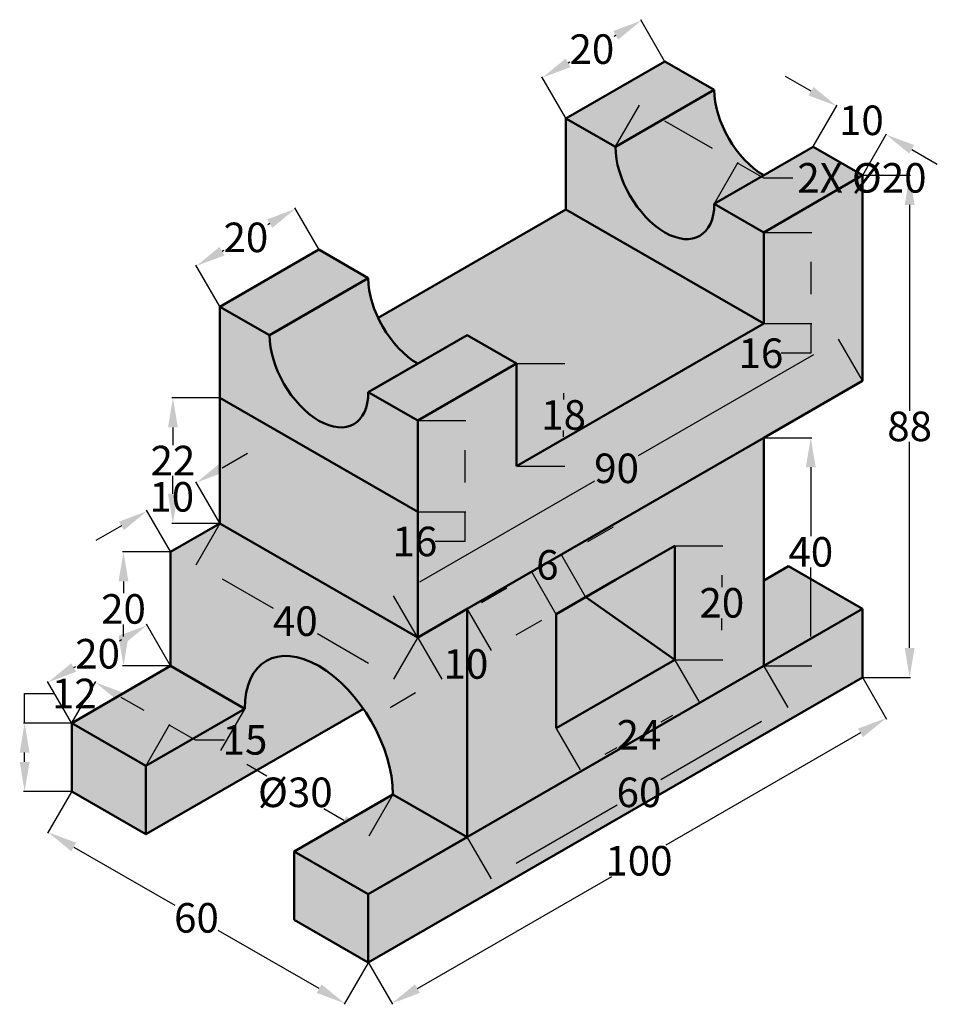
# Model space of a CAD drawing. Units: millimetres. Extents: x 125 to 286, y 8 to 181.
import ezdxf

# ---------------------------------------------------------------- set-up
doc = ezdxf.new("R2010")
doc.units = ezdxf.units.MM
doc.header["$MEASUREMENT"] = 0
for name, color, linetype, lineweight in [('M-DIMS', 2, 'Continuous', 18), ('M-HATC', 252, 'Continuous', 18), ('M-OUTL', 7, 'Continuous', 50)]:
    doc.layers.add(name, color=color, linetype=linetype, lineweight=lineweight)
doc.styles.get("Standard").update_dxf_attribs({"font": 'arial.ttf'})
doc.dimstyles.get("Standard").update_dxf_attribs({"dimtxt": 5.179999999999999, "dimasz": 5.179999999999999, "dimexe": 0.18, "dimexo": 0.0625, "dimgap": 0.09, "dimtad": 0, "dimtih": 1, "dimtoh": 1, "dimdec": 1, "dimzin": 0, "dimdsep": 46, "dimtxsty": 'Standard', "dimcen": 0.09, "dimadec": 0, "dimazin": 0, "dimtfac": 1, "dimtdec": 1, "dimtofl": 0, "dimtmove": 0, "dimatfit": 3, "dimfxl": 1, "dimtolj": 1, "dimtzin": 0, "dimarcsym": 0})

# ---------------------------------------------------------------- blocks, each defined once
blk = doc.blocks.new('*D1')
at = {"layer": 'Defpoints', "color": 0, "transparency": 16777216}
for p in [(272.9292849999999, 65.249038), (186.326745, 15.24903799999998), (190.4517447010181, 8.104328936630097)]:
    blk.add_point(p, dxfattribs=at)
at = {"layer": 'M-DIMS', "color": 0, "lineweight": -2, "transparency": 16777216}
for p, q in [((272.9605349999999, 65.19491141226347), (277.1442847956291, 57.94844420007783)), ((272.5682732040257, 55.51432877275904), (238.489772003563, 35.83909693109291)), ((194.9377562926215, 10.6943289366301), (229.0162574930842, 30.36956077829619)), ((186.3579949999999, 15.19491141226346), (190.5417447010181, 7.94844436394888))]:
    blk.add_line(p, q, dxfattribs=at)
at = {"layer": 'M-DIMS', "color": 0, "transparency": 16777216}
for points in [[(272.1366065373591, 56.26199737135959), (272.9999398706924, 54.76666017415848), (277.0542847956291, 58.10432877275904)], [(194.5060896259549, 11.44199753523065), (195.3694229592882, 9.946660338029531), (190.4517447010181, 8.104328936630097)]]:
    blk.add_solid(points, dxfattribs=at)
at = {"layer": 'M-DIMS', "color": 0, "transparency": 16777216, "insert": (233.7530147483236, 33.10432885469456), "char_height": 5.179999999999999, "attachment_point": 5}
blk.add_mtext('\\A1;100', dxfattribs=at)
blk = doc.blocks.new('*D2')
at = {"layer": 'Defpoints', "color": 0, "transparency": 16777216}
for p in [(134.3652209999999, 45.24903799999999), (130.240221223293, 38.10432880553328), (186.326745, 15.24903800000001)]:
    blk.add_point(p, dxfattribs=at)
at = {"layer": 'M-DIMS', "color": 0, "lineweight": -2, "transparency": 16777216}
for p, q in [((134.3339709999999, 45.19491141226347), (130.150221223293, 37.94844423285206)), ((134.7262328148964, 35.51432880553328), (152.415587617297, 25.30137504857649)), ((177.7157336884562, 10.69432890385592), (160.0263788860555, 20.90728266081271)), ((186.2954949999999, 15.19491141226348), (182.1117452800596, 7.948444331174698))]:
    blk.add_line(p, q, dxfattribs=at)
at = {"layer": 'M-DIMS', "color": 0, "transparency": 16777216}
for points in [[(135.157899481563, 36.26199740413384), (134.2945661482297, 34.76666020693271), (130.240221223293, 38.10432880553328)], [(178.1474003551229, 11.44199750245647), (177.2840670217895, 9.94666030525535), (182.2017452800596, 8.104328903855915)]]:
    blk.add_solid(points, dxfattribs=at)
at = {"layer": 'M-DIMS', "color": 0, "transparency": 16777216, "insert": (156.2209832516763, 23.1043288546946), "char_height": 5.179999999999999, "attachment_point": 5}
blk.add_mtext('\\A1;60', dxfattribs=at)
blk = doc.blocks.new('*D3')
at = {"layer": 'Defpoints', "color": 0, "transparency": 16777216}
for p in [(134.365221, 57.24903799999999), (151.4806020634321, 56.89374769108934), (147.355602, 49.74903799999999)]:
    blk.add_point(p, dxfattribs=at)
at = {"layer": 'M-DIMS', "color": 0, "lineweight": -2, "transparency": 16777216}
for p, q in [((134.396471, 57.30316458773652), (138.5802210492405, 64.54963223918992)), ((142.9762326408438, 61.80374766650871), (146.9945904718287, 59.48374769108935)), ((147.386852, 49.80316458773652), (151.5706020634322, 57.04963226377056)), ((151.4806020634321, 56.89374769108934), (155.9666136550356, 54.30374769108934)), ((155.9666136550356, 54.30374769108934), (161.1466136550355, 54.30374769108937))]:
    blk.add_line(p, q, dxfattribs=at)
at = {"layer": 'M-DIMS', "color": 0, "transparency": 16777216}
for points in [[(143.4078993075105, 62.55141626510927), (142.5445659741772, 61.05607906790815), (138.4902210492405, 64.3937476665087)], [(147.4262571384954, 60.23141628968992), (146.5629238051621, 58.73607909248879), (151.4806020634321, 56.89374769108934)]]:
    blk.add_solid(points, dxfattribs=at)
at = {"layer": 'M-DIMS', "color": 0, "transparency": 16777216, "insert": (164.7223367109701, 54.30374769108935), "char_height": 5.179999999999999, "attachment_point": 5}
blk.add_mtext('\\A1;15', dxfattribs=at)
blk = doc.blocks.new('*D4')
at = {"layer": 'Defpoints', "color": 0, "transparency": 16777216}
for p in [(126.1152210000001, 57.24903800000003), (134.365221, 57.24903800000003), (134.365221, 45.24903800000001)]:
    blk.add_point(p, dxfattribs=at)
at = {"layer": 'M-DIMS', "color": 0, "lineweight": -2, "transparency": 16777216}
for p, q in [((126.1152210000001, 57.24903800000003), (126.1152210000001, 62.42903800000003)), ((126.1152210000001, 62.42903800000003), (131.2952210000001, 62.42903800000003)), ((134.302721, 57.24903800000003), (125.9352210000001, 57.24903800000003)), ((126.1152210000001, 50.42903800000002), (126.1152210000001, 52.06903800000002)), ((134.302721, 45.24903800000001), (125.9352210000001, 45.24903800000001))]:
    blk.add_line(p, q, dxfattribs=at)
at = {"layer": 'M-DIMS', "color": 0, "transparency": 16777216}
for points in [[(125.2518876666668, 52.06903800000002), (126.9785543333334, 52.06903800000002), (126.1152210000001, 57.24903800000003)], [(125.2518876666668, 50.42903800000002), (126.9785543333334, 50.42903800000002), (126.1152210000001, 45.24903800000001)]]:
    blk.add_solid(points, dxfattribs=at)
at = {"layer": 'M-DIMS', "color": 0, "transparency": 16777216, "insert": (134.8250095402456, 62.42903799999997), "char_height": 5.179999999999999, "attachment_point": 5}
blk.add_mtext('\\A1;12', dxfattribs=at)
blk = doc.blocks.new('*D5')
at = {"layer": 'Defpoints', "color": 0, "transparency": 16777216}
for p in [(147.5607288281247, 74.39374787891832), (151.685729, 67.24903799999998), (134.365221, 57.24903799999999)]:
    blk.add_point(p, dxfattribs=at)
at = {"layer": 'M-DIMS', "color": 0, "lineweight": -2, "transparency": 16777216}
for p, q in [((151.654479, 67.30316458773653), (147.4707288281247, 74.5496324515995)), ((143.0747172365213, 71.80374787891832), (142.7359045594549, 71.60813428860915)), ((134.7262324008059, 66.98374791169252), (135.0650450778723, 67.17936150200165)), ((134.333971, 57.30316458773652), (130.1502208092025, 64.5496324843737))]:
    blk.add_line(p, q, dxfattribs=at)
at = {"layer": 'M-DIMS', "color": 0, "transparency": 16777216}
for points in [[(142.6430505698547, 72.55141647751887), (143.506383903188, 71.05607928031775), (147.5607288281247, 74.39374787891832)], [(134.2945657341392, 67.73141651029307), (135.1578990674726, 66.23607931309193), (130.2402208092025, 64.39374791169251)]]:
    blk.add_solid(points, dxfattribs=at)
at = {"layer": 'M-DIMS', "color": 0, "transparency": 16777216, "insert": (138.9004748186636, 69.39374789530541), "char_height": 5.179999999999999, "attachment_point": 5}
blk.add_mtext('\\A1;20', dxfattribs=at)
blk = doc.blocks.new('*D6')
at = {"layer": 'Defpoints', "color": 0, "transparency": 16777216}
for p in [(255.608777, 67.24903799999998), (203.647253, 37.24903799999998), (207.7722527199404, 30.1043289038559)]:
    blk.add_point(p, dxfattribs=at)
at = {"layer": 'M-DIMS', "color": 0, "lineweight": -2, "transparency": 16777216}
for p, q in [((255.640027, 67.19491141226347), (259.823776776707, 59.94844423285207)), ((255.2477651851035, 57.51432880553327), (237.5584103827029, 47.30137504857646)), ((212.2582643115437, 32.69432890385591), (229.9476191139444, 42.90728266081268)), ((203.678503, 37.19491141226346), (207.8622527199403, 29.9484443311747))]:
    blk.add_line(p, q, dxfattribs=at)
at = {"layer": 'M-DIMS', "color": 0, "transparency": 16777216}
for points in [[(254.8160985184368, 58.26199740413382), (255.6794318517702, 56.7666602069327), (259.7337767767069, 60.10432880553327)], [(211.8265976448771, 33.44199750245646), (212.6899309782104, 31.94666030525534), (207.7722527199404, 30.1043289038559)]]:
    blk.add_solid(points, dxfattribs=at)
at = {"layer": 'M-DIMS', "color": 0, "transparency": 16777216, "insert": (233.7530147483236, 45.10432885469458), "char_height": 5.179999999999999, "attachment_point": 5}
blk.add_mtext('\\A1;60', dxfattribs=at)
blk = doc.blocks.new('*D7')
at = {"layer": 'Defpoints', "color": 0, "transparency": 16777216}
for p in [(255.6087770000001, 107.249038), (255.6087770000001, 67.24903800000003), (263.8587770000002, 67.24903800000003)]:
    blk.add_point(p, dxfattribs=at)
at = {"layer": 'M-DIMS', "color": 0, "lineweight": -2, "transparency": 16777216}
for p, q in [((255.6712770000001, 107.249038), (264.0387770000002, 107.249038)), ((263.8587770000002, 102.069038), (263.8587770000002, 89.98380607639841)), ((263.8587770000002, 72.42903800000003), (263.8587770000002, 84.51426992360167)), ((255.6712770000001, 67.24903800000003), (264.0387770000002, 67.24903800000003))]:
    blk.add_line(p, q, dxfattribs=at)
at = {"layer": 'M-DIMS', "color": 0, "transparency": 16777216}
for points in [[(262.9954436666669, 102.069038), (264.7221103333336, 102.069038), (263.8587770000002, 107.249038)], [(262.9954436666669, 72.42903800000003), (264.7221103333336, 72.42903800000003), (263.8587770000002, 67.24903800000003)]]:
    blk.add_solid(points, dxfattribs=at)
at = {"layer": 'M-DIMS', "color": 0, "transparency": 16777216, "insert": (263.8587770000001, 87.24903799999996), "char_height": 5.179999999999999, "attachment_point": 5}
blk.add_mtext('\\A1;40', dxfattribs=at)
blk = doc.blocks.new('*D8')
at = {"layer": 'Defpoints', "color": 0, "transparency": 16777216}
for p in [(164.67611, 59.749038), (160.5511102374847, 52.60432883011397), (190.6568719999999, 44.74903799999998)]:
    blk.add_point(p, dxfattribs=at)
at = {"layer": 'M-DIMS', "color": 0, "lineweight": -2, "transparency": 16777216}
for p, q in [((164.64486, 59.69491141226347), (160.4611102374847, 52.44844425743277)), ((165.037121829088, 50.01432883011397), (168.5538111106856, 47.98396732672736)), ((190.6256219999999, 44.69491141226344), (186.4418722658679, 37.44844430659404)), ((182.0458606742645, 40.19432887927524), (178.529171392667, 42.22469038266187))]:
    blk.add_line(p, q, dxfattribs=at)
at = {"layer": 'M-DIMS', "color": 0, "transparency": 16777216}
for points in [[(165.4687884957547, 50.76199742871453), (164.6054551624214, 49.26666023151341), (160.5511102374847, 52.60432883011397)], [(182.4775273409312, 40.9419974778758), (181.6141940075979, 39.44666028067468), (186.5318722658679, 37.60432887927525)]]:
    blk.add_solid(points, dxfattribs=at)
at = {"layer": 'M-DIMS', "color": 0, "transparency": 16777216, "insert": (173.5414912516763, 45.10432885469461), "char_height": 5.179999999999999, "attachment_point": 5}
blk.add_mtext('\\A1;%%c30', dxfattribs=at)
blk = doc.blocks.new('*D9')
at = {"layer": 'Defpoints', "color": 0, "transparency": 16777216}
for p in [(240.0203199999999, 68.32469), (219.23571, 56.32469), (223.360710219983, 49.17998003775657)]:
    blk.add_point(p, dxfattribs=at)
at = {"layer": 'M-DIMS', "color": 0, "lineweight": -2, "transparency": 16777216}
for p, q in [((240.05157, 68.27056341226347), (244.2353201426896, 61.0240955989514)), ((239.6593085510863, 58.5899801716326), (237.5866782099857, 57.39334648626763)), ((219.26696, 56.27056341226347), (223.450710219983, 49.02409546507538)), ((227.8467218115864, 51.76998003775658), (229.9193521526869, 52.96661372312155))]:
    blk.add_line(p, q, dxfattribs=at)
at = {"layer": 'M-DIMS', "color": 0, "transparency": 16777216}
for points in [[(239.2276418844196, 59.33764877023317), (240.0909752177529, 57.84231157303204), (244.1453201426896, 61.17998017163261)], [(227.4150551449198, 52.51764863635714), (228.2783884782531, 51.02231143915602), (223.360710219983, 49.17998003775657)]]:
    blk.add_solid(points, dxfattribs=at)
at = {"layer": 'M-DIMS', "color": 0, "transparency": 16777216, "insert": (233.7530151813363, 55.17998010469459), "char_height": 5.179999999999999, "attachment_point": 5}
blk.add_mtext('\\A1;24', dxfattribs=at)
blk = doc.blocks.new('*D10')
at = {"layer": 'Defpoints', "color": 0, "transparency": 16777216}
for p in [(240.0203200000001, 88.32469000000003), (240.0203200000001, 68.32469000000003), (248.2703200000002, 68.32469000000003)]:
    blk.add_point(p, dxfattribs=at)
at = {"layer": 'M-DIMS', "color": 0, "lineweight": -2, "transparency": 16777216}
for p, q in [((240.0828200000001, 88.32469000000003), (248.4503200000002, 88.32469000000003)), ((248.2703200000002, 83.14469000000004), (248.2703200000002, 81.05945807639839)), ((248.2703200000002, 73.50469000000002), (248.2703200000002, 75.58992192360166)), ((240.0828200000001, 68.32469000000003), (248.4503200000002, 68.32469000000003))]:
    blk.add_line(p, q, dxfattribs=at)
at = {"layer": 'M-DIMS', "color": 0, "transparency": 16777216}
for points in [[(247.4069866666669, 83.14469000000004), (249.1336533333336, 83.14469000000004), (248.2703200000002, 88.32469000000003)], [(247.4069866666669, 73.50469000000002), (249.1336533333336, 73.50469000000002), (248.2703200000002, 68.32469000000003)]]:
    blk.add_solid(points, dxfattribs=at)
at = {"layer": 'M-DIMS', "color": 0, "transparency": 16777216, "insert": (248.2703200000002, 78.32468999999995), "char_height": 5.179999999999999, "attachment_point": 5}
blk.add_mtext('\\A1;20', dxfattribs=at)
blk = doc.blocks.new('*D11')
at = {"layer": 'Defpoints', "color": 0, "transparency": 16777216}
for p in [(268.8042848612385, 124.3937478215634), (272.929285, 117.249038), (194.986999, 72.24903799999998)]:
    blk.add_point(p, dxfattribs=at)
at = {"layer": 'M-DIMS', "color": 0, "lineweight": -2, "transparency": 16777216}
for p, q in [((272.898035, 117.3031645877365), (268.7142848612386, 124.5496323942446)), ((264.3182732696351, 121.8037478215634), (233.6244037559079, 104.0826339953417)), ((195.3480103676921, 81.98374796904739), (226.0418798814194, 99.70486179526908)), ((194.9557489999999, 72.30316458773652), (190.7719987760886, 79.54963254172857))]:
    blk.add_line(p, q, dxfattribs=at)
at = {"layer": 'M-DIMS', "color": 0, "transparency": 16777216}
for points in [[(263.8866066029685, 122.551416420164), (264.7499399363018, 121.0560792229628), (268.8042848612385, 124.3937478215634)], [(194.9163437010254, 82.73141656764794), (195.7796770343587, 81.23607937044682), (190.8619987760887, 79.39374796904738)]]:
    blk.add_solid(points, dxfattribs=at)
at = {"layer": 'M-DIMS', "color": 0, "transparency": 16777216, "insert": (229.8331418186636, 101.8937478953054), "char_height": 5.179999999999999, "attachment_point": 5}
blk.add_mtext('\\A1;90', dxfattribs=at)
blk = doc.blocks.new('*D12')
at = {"layer": 'Defpoints', "color": 0, "transparency": 16777216}
for p in [(160.346003, 92.24902699999998), (156.2210028978176, 85.10431724179332), (194.986999, 72.24903799999998)]:
    blk.add_point(p, dxfattribs=at)
at = {"layer": 'M-DIMS', "color": 0, "lineweight": -2, "transparency": 16777216}
for p, q in [((160.314753, 92.19490041226345), (156.1310028978176, 84.94843266911212)), ((160.707014489421, 82.51431724179334), (169.6460030815547, 77.35338977184198)), ((186.3759875809189, 67.6943287175958), (177.4369989887852, 72.85525618754716)), ((194.9557489999999, 72.19491141226345), (190.7719991725223, 64.94844414491459))]:
    blk.add_line(p, q, dxfattribs=at)
at = {"layer": 'M-DIMS', "color": 0, "transparency": 16777216}
for points in [[(161.1386811560877, 83.2619858403939), (160.2753478227543, 81.76664864319277), (156.2210028978176, 85.10431724179332)], [(186.8076542475855, 68.44199731619636), (185.9443209142522, 66.94666011899523), (190.8619991725223, 65.10432871759579)]]:
    blk.add_solid(points, dxfattribs=at)
at = {"layer": 'M-DIMS', "color": 0, "transparency": 16777216, "insert": (173.5415010351699, 75.10432297969454), "char_height": 5.179999999999999, "attachment_point": 5}
blk.add_mtext('\\A1;40', dxfattribs=at)
blk = doc.blocks.new('*D13')
at = {"layer": 'Defpoints', "color": 0, "transparency": 16777216}
for p in [(143.4357290000001, 87.24901500000003), (151.685729, 87.24901500000003), (151.685729, 67.24903800000003)]:
    blk.add_point(p, dxfattribs=at)
at = {"layer": 'M-DIMS', "color": 0, "lineweight": -2, "transparency": 16777216}
for p, q in [((151.623229, 87.24901500000003), (143.2557290000001, 87.24901500000003)), ((143.4357290000001, 82.06901500000002), (143.4357290000001, 79.9837945763984)), ((143.4357290000001, 72.42903800000003), (143.4357290000001, 74.51425842360166)), ((151.623229, 67.24903800000003), (143.2557290000001, 67.24903800000003))]:
    blk.add_line(p, q, dxfattribs=at)
at = {"layer": 'M-DIMS', "color": 0, "transparency": 16777216}
for points in [[(142.5723956666668, 82.06901500000002), (144.2990623333334, 82.06901500000002), (143.4357290000001, 87.24901500000003)], [(142.5723956666668, 72.42903800000003), (144.2990623333334, 72.42903800000003), (143.4357290000001, 67.24903800000003)]]:
    blk.add_solid(points, dxfattribs=at)
at = {"layer": 'M-DIMS', "color": 0, "transparency": 16777216, "insert": (143.4357290000001, 77.24902649999997), "char_height": 5.179999999999999, "attachment_point": 5}
blk.add_mtext('\\A1;20', dxfattribs=at)
blk = doc.blocks.new('*D14')
at = {"layer": 'Defpoints', "color": 0, "transparency": 16777216}
for p in [(152.0960030000001, 114.249027), (160.346003, 114.249027), (160.346003, 92.24902700000003)]:
    blk.add_point(p, dxfattribs=at)
at = {"layer": 'M-DIMS', "color": 0, "lineweight": -2, "transparency": 16777216}
for p, q in [((160.283503, 114.249027), (151.9160030000001, 114.249027)), ((152.0960030000001, 109.069027), (152.0960030000001, 105.9396272728513)), ((152.0960030000001, 97.429027), (152.0960030000001, 100.5584267271487)), ((160.283503, 92.24902700000003), (151.9160030000001, 92.24902700000001))]:
    blk.add_line(p, q, dxfattribs=at)
at = {"layer": 'M-DIMS', "color": 0, "transparency": 16777216}
for points in [[(151.2326696666668, 109.069027), (152.9593363333334, 109.069027), (152.0960030000001, 114.249027)], [(151.2326696666668, 97.429027), (152.9593363333334, 97.429027), (152.0960030000001, 92.24902700000001)]]:
    blk.add_solid(points, dxfattribs=at)
at = {"layer": 'M-DIMS', "color": 0, "transparency": 16777216, "insert": (152.0960030000001, 103.2490269999999), "char_height": 5.179999999999999, "attachment_point": 5}
blk.add_mtext('\\A1;22', dxfattribs=at)
blk = doc.blocks.new('*D15')
at = {"layer": 'Defpoints', "color": 0, "transparency": 16777216}
for p in [(194.9869990000001, 110.249038), (194.9869990000001, 94.24903800000001), (203.2369990000002, 94.24903800000001)]:
    blk.add_point(p, dxfattribs=at)
at = {"layer": 'M-DIMS', "color": 0, "lineweight": -2, "transparency": 16777216}
for p, q in [((195.0494990000001, 110.249038), (203.4169990000002, 110.249038)), ((203.2369990000002, 105.069038), (203.2369990000002, 99.42903800000003)), ((195.0494990000001, 94.24903800000001), (203.4169990000002, 94.24903800000001)), ((203.2369990000002, 94.24903800000001), (203.2369990000002, 89.06903800000002)), ((203.2369990000002, 89.06903800000002), (198.0569990000002, 89.06903800000002))]:
    blk.add_line(p, q, dxfattribs=at)
at = {"layer": 'M-DIMS', "color": 0, "transparency": 16777216}
for points in [[(202.3736656666669, 105.069038), (204.1003323333336, 105.069038), (203.2369990000002, 110.249038)], [(202.3736656666669, 99.42903800000003), (204.1003323333336, 99.42903800000003), (203.2369990000002, 94.24903800000001)]]:
    blk.add_solid(points, dxfattribs=at)
at = {"layer": 'M-DIMS', "color": 0, "transparency": 16777216, "insert": (194.5024764897683, 89.06903799999994), "char_height": 5.179999999999999, "attachment_point": 5}
blk.add_mtext('\\A1;16', dxfattribs=at)
blk = doc.blocks.new('*D16')
at = {"layer": 'Defpoints', "color": 0, "transparency": 16777216}
for p in [(212.3075070000001, 120.249038), (212.3075070000001, 102.249038), (220.5575070000002, 102.249038)]:
    blk.add_point(p, dxfattribs=at)
at = {"layer": 'M-DIMS', "color": 0, "lineweight": -2, "transparency": 16777216}
for p, q in [((212.3700070000001, 120.249038), (220.7375070000002, 120.249038)), ((220.5575070000002, 115.069038), (220.5575070000002, 113.9838060763984)), ((220.5575070000002, 107.429038), (220.5575070000002, 108.5142699236017)), ((212.3700070000001, 102.249038), (220.7375070000002, 102.249038))]:
    blk.add_line(p, q, dxfattribs=at)
at = {"layer": 'M-DIMS', "color": 0, "transparency": 16777216}
for points in [[(219.6941736666669, 115.069038), (221.4208403333336, 115.069038), (220.5575070000002, 120.249038)], [(219.6941736666669, 107.429038), (221.4208403333336, 107.429038), (220.5575070000002, 102.249038)]]:
    blk.add_solid(points, dxfattribs=at)
at = {"layer": 'M-DIMS', "color": 0, "transparency": 16777216, "insert": (220.5575070000002, 111.2490379999999), "char_height": 5.179999999999999, "attachment_point": 5}
blk.add_mtext('\\A1;18', dxfattribs=at)
blk = doc.blocks.new('*D17')
at = {"layer": 'Defpoints', "color": 0, "transparency": 16777216}
for p in [(173.5415108281247, 147.3719848789183), (177.666511, 140.227275), (160.3460029999999, 130.2272749999999)]:
    blk.add_point(p, dxfattribs=at)
at = {"layer": 'M-DIMS', "color": 0, "lineweight": -2, "transparency": 16777216}
for p, q in [((177.635261, 140.2814015877365), (173.4515108281247, 147.5278694515995)), ((169.0554992365213, 144.7819848789183), (168.7166865594549, 144.5863712886091)), ((160.7070144008059, 139.9619849116925), (161.0458270778723, 140.1575985020016)), ((160.314753, 130.2814015877365), (156.1310028092025, 137.5278694843737))]:
    blk.add_line(p, q, dxfattribs=at)
at = {"layer": 'M-DIMS', "color": 0, "transparency": 16777216}
for points in [[(168.6238325698547, 145.5296534775188), (169.487165903188, 144.0343162803177), (173.5415108281247, 147.3719848789183)], [(160.2753477341392, 140.709653510293), (161.1386810674726, 139.2143163130919), (156.2210028092025, 137.3719849116925)]]:
    blk.add_solid(points, dxfattribs=at)
at = {"layer": 'M-DIMS', "color": 0, "transparency": 16777216, "insert": (164.8812568186636, 142.3719848953053), "char_height": 5.179999999999999, "attachment_point": 5}
blk.add_mtext('\\A1;20', dxfattribs=at)
blk = doc.blocks.new('*D18')
at = {"layer": 'Defpoints', "color": 0, "transparency": 16777216}
for p in [(234.1632898281247, 180.3719848789182), (238.28829, 173.2272749999999), (220.967782, 163.2272749999999)]:
    blk.add_point(p, dxfattribs=at)
at = {"layer": 'M-DIMS', "color": 0, "lineweight": -2, "transparency": 16777216}
for p, q in [((238.25704, 173.2814015877364), (234.0732898281247, 180.5278694515994)), ((229.6772782365213, 177.7819848789182), (229.3384655594548, 177.586371288609)), ((221.3287934008059, 172.9619849116925), (221.6676060778723, 173.1575985020016)), ((220.936532, 163.2814015877365), (216.7527818092025, 170.5278694843737))]:
    blk.add_line(p, q, dxfattribs=at)
at = {"layer": 'M-DIMS', "color": 0, "transparency": 16777216}
for points in [[(229.2456115698546, 178.5296534775188), (230.108944903188, 177.0343162803177), (234.1632898281247, 180.3719848789182)], [(220.8971267341393, 173.709653510293), (221.7604600674726, 172.2143163130919), (216.8427818092025, 170.3719849116925)]]:
    blk.add_solid(points, dxfattribs=at)
at = {"layer": 'M-DIMS', "color": 0, "transparency": 16777216, "insert": (225.5030358186636, 175.3719848953053), "char_height": 5.179999999999999, "attachment_point": 5}
blk.add_mtext('\\A1;20', dxfattribs=at)
blk = doc.blocks.new('*D19')
at = {"layer": 'Defpoints', "color": 0, "transparency": 16777216}
for p in [(255.6087770000001, 143.249038), (255.6087770000001, 127.249038), (263.8587770000003, 127.249038)]:
    blk.add_point(p, dxfattribs=at)
at = {"layer": 'M-DIMS', "color": 0, "lineweight": -2, "transparency": 16777216}
for p, q in [((255.6712770000001, 143.249038), (264.0387770000002, 143.249038)), ((263.8587770000002, 138.069038), (263.8587770000002, 132.429038)), ((255.6712770000001, 127.249038), (264.0387770000003, 127.249038)), ((263.8587770000003, 127.249038), (263.8587770000003, 122.069038)), ((263.8587770000003, 122.069038), (258.6787770000003, 122.069038))]:
    blk.add_line(p, q, dxfattribs=at)
at = {"layer": 'M-DIMS', "color": 0, "transparency": 16777216}
for points in [[(262.9954436666669, 138.069038), (264.7221103333336, 138.069038), (263.8587770000002, 143.249038)], [(262.9954436666669, 132.429038), (264.7221103333336, 132.429038), (263.8587770000003, 127.249038)]]:
    blk.add_solid(points, dxfattribs=at)
at = {"layer": 'M-DIMS', "color": 0, "transparency": 16777216, "insert": (255.1242544897683, 122.0690379999999), "char_height": 5.179999999999999, "attachment_point": 5}
blk.add_mtext('\\A1;16', dxfattribs=at)
blk = doc.blocks.new('*D20')
at = {"layer": 'Defpoints', "color": 0, "transparency": 16777216}
for p in [(277.0542851860669, 160.3937479034989), (264.269031, 158.249038), (272.929285, 153.249038)]:
    blk.add_point(p, dxfattribs=at)
at = {"layer": 'M-DIMS', "color": 0, "lineweight": -2, "transparency": 16777216}
for p, q in [((263.9080195850024, 167.9837478871118), (259.422007993399, 170.5737478871119)), ((264.300281, 158.3031645877365), (268.4840311766059, 165.549632459793)), ((272.960535, 153.3031645877365), (277.1442851860669, 160.5496324761801)), ((281.5402967776703, 157.8037479034989), (286.0263083692737, 155.2137479034988))]:
    blk.add_line(p, q, dxfattribs=at)
at = {"layer": 'M-DIMS', "color": 0, "transparency": 16777216}
for points in [[(264.3396862516691, 168.7314164857124), (263.4763529183357, 167.2360792885113), (268.3940311766058, 165.3937478871118)], [(281.971963444337, 158.5514165020994), (281.1086301110036, 157.0560793048983), (277.0542851860669, 160.3937479034989)]]:
    blk.add_solid(points, dxfattribs=at)
at = {"layer": 'M-DIMS', "color": 0, "transparency": 16777216, "insert": (272.7241581813364, 162.8937478953053), "char_height": 5.179999999999999, "attachment_point": 5}
blk.add_mtext('\\A1;10', dxfattribs=at)
blk = doc.blocks.new('*D21')
at = {"layer": 'Defpoints', "color": 0, "transparency": 16777216}
for p in [(272.9292850000001, 153.249038), (281.1792850000001, 153.249038), (272.9292850000001, 65.24903800000003)]:
    blk.add_point(p, dxfattribs=at)
at = {"layer": 'M-DIMS', "color": 0, "lineweight": -2, "transparency": 16777216}
for p, q in [((272.9917850000001, 153.249038), (281.3592850000002, 153.249038)), ((281.1792850000001, 148.069038), (281.1792850000002, 111.9838060763984)), ((281.1792850000002, 70.42903800000003), (281.1792850000002, 106.5142699236017)), ((272.9917850000001, 65.24903800000003), (281.3592850000002, 65.24903800000003))]:
    blk.add_line(p, q, dxfattribs=at)
at = {"layer": 'M-DIMS', "color": 0, "transparency": 16777216}
for points in [[(280.3159516666668, 148.069038), (282.0426183333335, 148.069038), (281.1792850000001, 153.249038)], [(280.3159516666669, 70.42903800000003), (282.0426183333335, 70.42903800000003), (281.1792850000002, 65.24903800000003)]]:
    blk.add_solid(points, dxfattribs=at)
at = {"layer": 'M-DIMS', "color": 0, "transparency": 16777216, "insert": (281.1792850000001, 109.2490379999999), "char_height": 5.179999999999999, "attachment_point": 5}
blk.add_mtext('\\A1;88', dxfattribs=at)
blk = doc.blocks.new('*D22')
at = {"layer": 'Defpoints', "color": 0, "transparency": 16777216}
for p in [(229.628015, 158.249038), (251.0735231907974, 155.3937479116925), (246.948523, 148.2490379999999)]:
    blk.add_point(p, dxfattribs=at)
at = {"layer": 'M-DIMS', "color": 0, "lineweight": -2, "transparency": 16777216}
for p, q in [((229.659265, 158.3031645877365), (233.8430151718752, 165.5496324515995)), ((238.2390267634786, 162.8037478789182), (246.587511599194, 157.9837479116925)), ((246.9797729999999, 148.3031645877365), (251.1635231907974, 155.5496324843737)), ((251.0735231907974, 155.3937479116925), (255.5595347824008, 152.8037479116925)), ((255.5595347824008, 152.8037479116925), (260.7395347824008, 152.8037479116925))]:
    blk.add_line(p, q, dxfattribs=at)
at = {"layer": 'M-DIMS', "color": 0, "transparency": 16777216}
for points in [[(238.6706934301453, 163.5514164775189), (237.8073600968119, 162.0560792803177), (233.7530151718752, 165.3937478789182)], [(247.0191782658607, 158.7314165102931), (246.1558449325273, 157.2360793130919), (251.0735231907974, 155.3937479116925)]]:
    blk.add_solid(points, dxfattribs=at)
at = {"layer": 'M-DIMS', "color": 0, "transparency": 16777216, "insert": (272.8202100893585, 152.8037479116925), "char_height": 5.179999999999999, "attachment_point": 5}
blk.add_mtext('\\A1;2X %%c20', dxfattribs=at)
blk = doc.blocks.new('*D23')
at = {"layer": 'Defpoints', "color": 0, "transparency": 16777216}
for p in [(156.2210033544831, 99.39373596723891), (160.346003, 92.24902700000001), (151.685729, 87.24901499999999)]:
    blk.add_point(p, dxfattribs=at)
at = {"layer": 'M-DIMS', "color": 0, "lineweight": -2, "transparency": 16777216}
for p, q in [((160.7070149460865, 101.9837359672389), (165.1930265376899, 104.5737359672389)), ((160.314753, 92.30315358773653), (156.1310033544831, 99.54962053992011)), ((151.654479, 87.30314158773653), (147.4707291488695, 94.54960889605317)), ((143.0747175572662, 91.80372432337197), (138.5887059656627, 89.21372432337198))]:
    blk.add_line(p, q, dxfattribs=at)
at = {"layer": 'M-DIMS', "color": 0, "transparency": 16777216}
for points in [[(160.2753482794198, 102.7314045658394), (161.1386816127532, 101.2360673686383), (156.2210033544831, 99.39373596723891)], [(142.6430508905995, 92.55139292197254), (143.5063842239328, 91.0560557247714), (147.5607291488695, 94.39372432337197)]]:
    blk.add_solid(points, dxfattribs=at)
at = {"layer": 'M-DIMS', "color": 0, "transparency": 16777216, "insert": (151.8908662516763, 96.89373014530545), "char_height": 5.179999999999999, "attachment_point": 5}
blk.add_mtext('\\A1;10', dxfattribs=at)
blk = doc.blocks.new('*D24')
at = {"layer": 'Defpoints', "color": 0, "transparency": 16777216}
for p in [(203.647253, 77.24903799999998), (194.986999, 72.24903799999998), (199.1119987435931, 65.10432886288814)]:
    blk.add_point(p, dxfattribs=at)
at = {"layer": 'M-DIMS', "color": 0, "lineweight": -2, "transparency": 16777216}
for p, q in [((203.678503, 77.19491141226347), (207.8622527530542, 69.94844427381985)), ((212.2582643446576, 72.69432884650104), (216.744275936261, 75.28432884650104)), ((195.018249, 72.19491141226347), (199.2019987435931, 64.94844429020694)), ((194.6259871519897, 62.51432886288813), (190.1399755603863, 59.92432886288813))]:
    blk.add_line(p, q, dxfattribs=at)
at = {"layer": 'M-DIMS', "color": 0, "transparency": 16777216}
for points in [[(211.8265976779909, 73.4419974451016), (212.6899310113242, 71.94666024790047), (207.7722527530542, 70.10432884650103)], [(194.194320485323, 63.26199746148869), (195.0576538186564, 61.76666026428756), (199.1119987435931, 65.10432886288814)]]:
    blk.add_solid(points, dxfattribs=at)
at = {"layer": 'M-DIMS', "color": 0, "transparency": 16777216, "insert": (203.4421257483236, 67.60432885469459), "char_height": 5.179999999999999, "attachment_point": 5}
blk.add_mtext('\\A1;10', dxfattribs=at)
blk = doc.blocks.new('*D25')
at = {"layer": 'Defpoints', "color": 0, "transparency": 16777216}
for p in [(220.306862871502, 86.46939980378673), (224.4318629999999, 79.32469), (219.23571, 76.32469)]:
    blk.add_point(p, dxfattribs=at)
at = {"layer": 'M-DIMS', "color": 0, "lineweight": -2, "transparency": 16777216}
for p, q in [((224.7928744631053, 89.05939980378675), (229.2788860547087, 91.64939980378674)), ((224.400613, 79.37881658773654), (220.2168628715019, 86.62528437646793)), ((219.20446, 76.37881658773652), (215.0207100158253, 83.62528412649256)), ((210.6246984242219, 80.87939955381134), (206.1386868326185, 78.28939955381132))]:
    blk.add_line(p, q, dxfattribs=at)
at = {"layer": 'M-DIMS', "color": 0, "transparency": 16777216}
for points in [[(224.3612077964387, 89.80706840238729), (225.224541129772, 88.31173120518618), (220.306862871502, 86.46939980378673)], [(210.1930317575552, 81.62706815241191), (211.0563650908886, 80.13173095521078), (215.1107100158253, 83.46939955381136)]]:
    blk.add_solid(points, dxfattribs=at)
at = {"layer": 'M-DIMS', "color": 0, "transparency": 16777216, "insert": (217.7087864436636, 84.96939967879904), "char_height": 5.179999999999999, "attachment_point": 5}
blk.add_mtext('\\A1;6', dxfattribs=at)

msp = doc.modelspace()

# ---------------------------------------------------------------- hatches: boundary and pattern name
at = {"layer": 'M-HATC'}
h = msp.add_hatch(color=256, dxfattribs=at)
h.dxf.hatch_style = 1
h.set_gradient(color1=(99, 100, 102), tint=1, name='INVHEMISPHERICAL')
edge = h.paths.add_edge_path()
edge.add_line((160.3460033766522, 92.2490266351085), (151.6857288522489, 87.24901480718822))
edge.add_line((151.6857288522489, 87.24901480718822), (151.6857288522489, 67.24903846302868))
edge.add_line((151.6857288522489, 67.2490384630287), (164.6761099090155, 59.74903846302871))
edge.add_ellipse((177.6664909657821, 52.2490384630287), major_axis=(9.185586535436917, -15.90990257669732), ratio=0.577350269189626, start_angle=103.89788624801389, end_angle=210, ccw=False)
edge.add_ellipse((177.6664909657821, 52.2490384630287), major_axis=(9.185586535436917, -15.90990257669732), ratio=0.577350269189626, start_angle=30, end_angle=103.89788624801389, ccw=False)
edge.add_line((190.6568720225486, 44.74903846302871), (192.28876578158, 43.80686416196308))
edge.add_line((192.28876578158, 43.80686416196307), (203.6472530793152, 37.2490384630287))
edge.add_line((203.6472530793152, 37.24903846302871), (203.6472530793152, 77.24903846302871))
edge.add_line((203.6472530793152, 77.24903846302871), (194.9869990414709, 72.24903846302875))
edge.add_line((194.9869990414709, 72.24903846302875), (160.3460033766522, 92.2490266351085))
h.paths.add_polyline_path([(164.6761099090155, 59.74903846302869), (151.6857288522489, 67.2490384630287), (134.3652207765601, 57.2490384630287), (147.3556018333267, 49.7490384630287)])
h.paths.add_polyline_path([(147.3556018333267, 49.74903846302869), (134.3652207765601, 57.24903846302869), (134.3652207765601, 45.24903846302871), (147.3556018333267, 37.74903846302871)])
h.paths.add_polyline_path([(272.9292853820703, 65.24903846302868), (272.9292853820703, 77.2490384630287), (186.3267450036264, 27.24903846302871), (186.3267450036264, 15.24903846302871)])
h.paths.add_polyline_path([(255.6087773063815, 67.24903846302868), (255.6087773063816, 107.2490384630287), (203.6472530793152, 77.24903846302871), (203.6472530793152, 37.24903846302871)])
h.paths.add_polyline_path([(219.2357103474352, 56.32469006310042), (219.2357103474352, 76.32469006310043), (229.6280151928484, 82.32469006310043), (240.0203200382617, 88.32469006310043), (240.0203200382617, 68.3246900631004)], flags=16)
h.paths.add_polyline_path([(240.0203200382617, 68.3246900631004), (224.4318627701418, 79.32469006310043), (219.2357103474352, 76.32469006310043), (219.2357103474352, 56.32469006310042)], flags=16)
h.paths.add_polyline_path([(255.6087773063816, 107.2490384630287), (272.9292853820704, 117.2490384630287), (272.9292853820704, 153.2490384630287), (255.6087773063817, 143.2490384630287), (255.6087773063817, 127.2490384630286), (212.3075071171597, 102.2490384630287), (212.3075071171597, 120.2490384630287), (194.9869990414709, 110.2490384630287), (194.9869990414709, 94.24903846302863), (194.9869990414709, 72.24903846302875), (203.6472530793152, 77.24903846302871)])
h.paths.add_polyline_path([(240.0203200382617, 88.32469006310043), (229.6280151928484, 82.32469006310043), (224.4318627701418, 79.32469006310043), (240.0203200382617, 68.3246900631004)], flags=0)
h.paths.add_polyline_path([(194.9869990414709, 94.24903846302864), (160.3460033766522, 114.2490266351084), (160.3460033766522, 92.2490266351085), (194.9869990414709, 72.24903846302875)])
edge = h.paths.add_edge_path()
edge.add_ellipse((194.986999041471, 130.2490384630287), major_axis=(6.123724356957941, -10.60660171779822), ratio=0.5773502691896263, start_angle=256.1022749873906, end_angle=329.99999999999983, ccw=False)
edge.add_ellipse((194.986999041471, 130.2490384630287), major_axis=(6.123724356957941, -10.60660171779822), ratio=0.5773502691896263, start_angle=210.1080463970273, end_angle=256.1022749873906, ccw=False)
edge.add_line((186.3267654901854, 135.2272753995162), (169.0062574144966, 125.2272753995162))
edge.add_ellipse((177.6664909657822, 120.2490384630287), major_axis=(6.123724356957941, -10.60660171779822), ratio=0.577350269189626, start_angle=210.1080463970272, end_angle=390)
edge.add_line((186.3267450036266, 115.2490384630286), (194.9869990414709, 120.2490384630287))
h.paths.add_polyline_path([(212.3075071171597, 120.2490384630287), (203.6472530793154, 125.2490384630287), (186.3267450036266, 115.2490384630286), (194.986999041471, 110.2490384630287)])
edge = h.paths.add_edge_path()
edge.add_line((194.9869990414709, 110.2490384630287), (186.3267450036266, 115.2490384630286))
edge.add_ellipse((177.6664909657822, 120.2490384630287), major_axis=(6.123724356957941, -10.60660171779822), ratio=0.577350269189626, start_angle=210.1080463970273, end_angle=390.00000000000006, ccw=False)
edge.add_line((169.0062574144966, 125.2272753995162), (160.3460033766522, 130.2272753995162))
edge.add_line((160.3460033766522, 130.2272753995162), (160.3460033766522, 114.2490266351084))
edge.add_line((160.3460033766522, 114.2490266351084), (194.9869990414709, 94.24903846302864))
edge.add_line((194.9869990414709, 94.24903846302864), (194.9869990414709, 110.2490384630287))
h.paths.add_polyline_path([(186.3267654901854, 135.2272753995162), (177.666511452341, 140.2272753995162), (160.3460033766522, 130.2272753995162), (169.0062574144966, 125.2272753995162)])
h.paths.add_polyline_path([(246.9485437550961, 168.2272753995163), (238.2882897172517, 173.2272753995162), (220.9677816415629, 163.2272753995162), (229.6280356794073, 158.2272753995162)])
edge = h.paths.add_edge_path()
edge.add_line((220.9677816415629, 147.2490266351084), (188.058804591158, 128.249019876302))
edge.add_ellipse((194.986999041471, 130.2490384630287), major_axis=(6.123724356957941, -10.60660171779822), ratio=0.5773502691896263, start_angle=256.1022749873905, end_angle=329.9999999999998)
edge.add_line((194.986999041471, 120.2490384630287), (203.6472530793154, 125.2490384630287))
edge.add_line((203.6472530793154, 125.2490384630287), (212.3075071171597, 120.2490384630287))
edge.add_line((212.3075071171597, 120.2490384630287), (212.3075071171597, 102.2490384630287))
edge.add_line((212.3075071171597, 102.2490384630287), (255.6087773063817, 127.2490384630287))
edge.add_line((255.6087773063817, 127.2490384630287), (220.9677816415629, 147.2490266351084))
edge = h.paths.add_edge_path()
edge.add_ellipse((255.6087773063817, 163.2490384630287), major_axis=(6.123724356957941, -10.60660171779822), ratio=0.577350269189626, start_angle=210.1080463970273, end_angle=329.9999999999999, ccw=False)
edge.add_line((246.9485437550961, 168.2272753995163), (229.6280356794073, 158.2272753995163))
edge.add_ellipse((238.2882692306929, 153.2490384630287), major_axis=(6.123724356957941, -10.60660171779822), ratio=0.5773502691896262, start_angle=210.1080463970272, end_angle=390.0000000000001)
edge.add_line((246.9485232685372, 148.2490384630287), (255.6087773063817, 153.2490384630287))
edge = h.paths.add_edge_path()
edge.add_line((229.6280356794073, 158.2272753995163), (220.9677816415629, 163.2272753995162))
edge.add_line((220.9677816415629, 163.2272753995162), (220.9677816415629, 147.2490266351085))
edge.add_line((220.9677816415629, 147.2490266351085), (255.6087773063816, 127.2490384630287))
edge.add_line((255.6087773063816, 127.2490384630287), (255.6087773063817, 143.2490384630287))
edge.add_line((255.6087773063817, 143.2490384630287), (246.9485232685373, 148.2490384630287))
edge.add_ellipse((238.2882692306929, 153.2490384630287), major_axis=(6.123724356957941, -10.60660171779822), ratio=0.5773502691896262, start_angle=210.1080463970273, end_angle=390.00000000000006, ccw=False)
h.paths.add_polyline_path([(272.9292853820705, 153.2490384630287), (264.2690313442261, 158.2490384630287), (246.9485232685373, 148.2490384630287), (255.6087773063817, 143.2490384630287)])
h.paths.add_polyline_path([(272.9292853820703, 77.24903846302868), (259.9389043253038, 84.74903846302868), (255.6087773063816, 82.20898283503291), (255.6087773063815, 67.24903846302868)])
h = msp.add_hatch(color=256, dxfattribs=at)
h.dxf.hatch_style = 1
h.paths.add_polyline_path([(240.0203200382617, 88.32469006310043), (229.6280151928484, 82.32469006310043), (224.4318627701418, 79.32469006310043), (240.0203200382617, 68.3246900631004)])
h = msp.add_hatch(color=256, dxfattribs=at)
h.dxf.hatch_style = 1
h.set_gradient(color1=(99, 100, 102), tint=1, name='CURVED')
edge = h.paths.add_edge_path()
edge.add_line((147.3556018333267, 49.74903846302871), (147.3556018333267, 37.74903846302871))
edge.add_line((147.3556018333267, 37.74903846302871), (185.460719599842, 59.74903846302869))
edge.add_ellipse((177.6664909657821, 52.2490384630287), major_axis=(9.185586535436917, -15.90990257669732), ratio=0.577350269189626, start_angle=103.8978862480139, end_angle=210)
edge.add_line((164.6761099090155, 59.7490384630287), (147.3556018333267, 49.74903846302871))
h = msp.add_hatch(color=256, dxfattribs=at)
h.dxf.hatch_style = 1
h.set_gradient(color1=(99, 100, 102), tint=1, name='CURVED')
h.paths.add_polyline_path([(190.6568720225486, 44.7490384630287), (173.3363639468598, 34.74903846302871), (186.3267450036264, 27.24903846302872), (203.6472530793152, 37.24903846302871)])
h.paths.add_polyline_path([(186.3267450036264, 27.24903846302872), (173.3363639468599, 34.74903846302871), (173.3363639468599, 22.74903846302871), (186.3267450036264, 15.24903846302871)])

# ---------------------------------------------------------------- linework, layer by layer
at = {"layer": 'M-OUTL'}
for p, q in [((220.9677816415629, 163.2272753995162), (238.2882897172517, 173.2272753995162)), ((238.2882897172517, 173.2272753995162), (246.9485437550961, 168.2272753995162)), ((246.9485437550961, 168.2272753995162), (229.6280356794073, 158.2272753995162)), ((229.6280356794073, 158.2272753995162), (220.9677816415629, 163.2272753995162)), ((220.9677816415629, 147.2490266351084), (220.9677816415629, 163.2272753995162)), ((246.9485232685373, 148.2490384630287), (264.2690313442261, 158.2490384630287)), ((264.2690313442261, 158.2490384630287), (272.9292853820704, 153.2490384630287)), ((272.9292853820704, 153.2490384630287), (255.6087773063817, 143.2490384630287)), ((272.9292853820704, 117.2490384630287), (272.9292853820704, 153.2490384630287)), ((220.9677816415629, 147.2490266351084), (188.058804591158, 128.249019876302)), ((255.6087773063817, 127.2490384630287), (220.9677816415629, 147.2490266351084)), ((255.6087773063817, 143.2490384630287), (246.9485232685373, 148.2490384630287)), ((255.6087773063817, 143.2490384630287), (255.6087773063817, 127.2490384630287)), ((160.3460033766522, 130.2272753995162), (177.666511452341, 140.2272753995162)), ((161.3822367933899, 130.825545041613), (177.666511452341, 140.2272753995162)), ((177.666511452341, 140.2272753995162), (186.3267654901854, 135.2272753995162)), ((186.3267654901854, 135.2272753995162), (169.0062574144966, 125.2272753995162)), ((186.3267654901854, 135.2272753995162), (170.0424908312343, 125.825545041613)), ((169.0062574144966, 125.2272753995162), (160.3460033766522, 130.2272753995162)), ((160.3460033766522, 114.2490266351084), (160.3460033766522, 130.2272753995162)), ((255.6087773063817, 127.2490384630287), (212.3075071171597, 102.2490384630287)), ((186.3267450036266, 115.2490384630286), (203.6472530793154, 125.2490384630287)), ((187.3629784203643, 115.8473081051255), (203.6472530793154, 125.2490384630286)), ((203.6472530793154, 125.2490384630287), (212.3075071171597, 120.2490384630287)), ((212.3075071171597, 120.2490384630287), (194.9869990414709, 110.2490384630287)), ((212.3075071171597, 120.2490384630287), (196.0232324582086, 110.8473081051255)), ((212.3075071171597, 102.2490384630286), (212.3075071171597, 120.2490384630287)), ((255.6087773063816, 107.2490384630287), (272.9292853820704, 117.2490384630287)), ((194.9869990414709, 94.24903846302864), (160.3460033766522, 114.2490266351084)), ((160.3460033766522, 114.2490266351084), (160.3460033766522, 92.2490266351085)), ((194.9869990414709, 110.2490384630287), (186.3267450036266, 115.2490384630286)), ((194.9869990414709, 110.2490384630287), (194.9869990414709, 94.24903846302863)), ((203.6472530793152, 77.24903846302871), (255.6087773063816, 107.2490384630287)), ((255.6087773063816, 107.2490384630287), (255.6087773063816, 67.2490384630287)), ((194.9869990414709, 95.72819089158182), (194.9869990414709, 72.24903846302875)), ((160.3460033766522, 92.2490266351085), (151.6857288522489, 87.24901480718822)), ((194.9869990414709, 72.24903846302875), (160.3460033766522, 92.2490266351085)), ((229.6280151928484, 82.32469006310043), (240.0203200382617, 88.32469006310043)), ((240.0203200382617, 88.32469006310043), (229.6280151928484, 82.32469006310043)), ((240.0203200382617, 68.3246900631004), (240.0203200382617, 88.32469006310043)), ((151.6857288522489, 67.2490384630287), (151.6857288522489, 87.24901480718822)), ((259.9389043253038, 84.74903846302868), (255.6087773063816, 82.20898283503291)), ((272.9292853820703, 77.2490384630287), (259.9389043253038, 84.74903846302868)), ((229.6280151928484, 82.32469006310043), (219.2357103474352, 76.32469006310043)), ((240.0203200382617, 68.3246900631004), (224.4318627701418, 79.32469006310043)), ((186.3267450036264, 27.24903846302871), (272.9292853820703, 77.2490384630287)), ((203.6472530793152, 77.24903846302871), (194.9869990414709, 72.24903846302875)), ((203.6472530793152, 37.24903846302871), (203.6472530793152, 77.24903846302871)), ((219.2357103474352, 76.32469006310043), (219.2357103474352, 56.32469006310043)), ((272.9292853820703, 77.2490384630287), (272.9292853820703, 65.2490384630287)), ((219.2357103474352, 56.32469006310043), (240.0203200382617, 68.3246900631004)), ((151.6857288522489, 67.2490384630287), (134.3652207765601, 57.2490384630287)), ((164.6761099090155, 59.7490384630287), (151.6857288522489, 67.2490384630287)), ((186.3267450036264, 15.24903846302871), (272.9292853820703, 65.2490384630287)), ((164.6761099090155, 59.74903846302869), (161.5389796193304, 61.56026148026132)), ((161.5389796193304, 61.56026148026132), (164.6761099090155, 59.7490384630287)), ((147.3556018333267, 49.74903846302871), (164.6761099090155, 59.7490384630287)), ((147.3556018333267, 37.74903846302871), (185.460719599842, 59.74903846302868)), ((147.3556018333267, 49.74903846302871), (134.3652207765601, 57.2490384630287)), ((134.3652207765601, 57.2490384630287), (134.3652207765601, 45.2490384630287)), ((147.3556018333267, 37.74903846302871), (147.3556018333267, 49.74903846302871)), ((134.3652207765601, 45.2490384630287), (147.3556018333267, 37.74903846302871)), ((190.6568720225486, 44.7490384630287), (173.3363639468599, 34.74903846302871)), ((203.6472530793152, 37.24903846302871), (190.6568720225486, 44.7490384630287)), ((190.6568720225486, 44.74903846302871), (192.28876578158, 43.80686416196307)), ((186.3267450036264, 27.24903846302872), (203.6472530793152, 37.24903846302871)), ((173.3363639468599, 34.74903846302871), (173.3363639468599, 22.74903846302871)), ((186.3267450036264, 27.24903846302872), (173.3363639468599, 34.74903846302871)), ((186.3267450036264, 15.24903846302871), (186.3267450036264, 27.24903846302871)), ((173.3363639468599, 22.74903846302871), (186.3267450036264, 15.24903846302871))]:
    msp.add_line(p, q, dxfattribs=at)
for centre, major_axis, ratio, start_param, end_param in [((255.6087773063817, 163.2490384630287), (6.123724356957941, -10.60660171779822), 0.5773502691896262, 3.929165942261613, 5.497787143782135), ((238.2882692306929, 153.2490384630287), (6.123724356957941, -10.60660171779822), 0.5773502691896262, 3.929165942261613, 7.068583470577035), ((194.986999041471, 130.2490384630287), (6.123724356957941, -10.60660171779822), 0.5773502691896262, 3.929165942261613, 5.497787143782135), ((177.6664909657822, 120.2490384630287), (6.123724356957941, -10.60660171779822), 0.5773502691896262, 3.929165942261613, 7.068583470577035), ((177.6664909657821, 52.2490384630287), (9.185586535436917, -15.90990257669732), 0.577350269189626, 0.7853981633974484, 3.926990816987241)]:
    msp.add_ellipse(centre, major_axis=major_axis, ratio=ratio, start_param=start_param, end_param=end_param, dxfattribs=at)

# ---------------------------------------------------------------- dimensions: what is measured, and where the dimension line sits
at = {"layer": 'M-DIMS'}
for base, p1, p2, angle, picture, middle in [((234.1632898281247, 180.3719848789182), (220.967782, 163.227275), (238.28829, 173.227275), 29.99999999999997, '*D18', (225.5030358186636, 175.3719848953053)), ((277.0542851860669, 160.3937479034989), (264.269031, 158.249038), (272.929285, 153.249038), 329.9999999999998, '*D20', (272.7241581813364, 162.8937478953053)), ((281.1792850000001, 153.249038), (272.929285, 65.249038), (272.929285, 153.249038), 90, '*D21', (281.1792850000001, 109.2490379999999)), ((173.5415108281247, 147.3719848789183), (160.346003, 130.227275), (177.666511, 140.227275), 29.99999999999993, '*D17', (164.8812568186636, 142.3719848953053)), ((263.8587770000003, 127.249038), (255.608777, 143.249038), (255.608777, 127.249038), 270, '*D19', (255.1242544897683, 122.0690379999999)), ((268.8042848612385, 124.3937478215634), (194.986999, 72.24903799999998), (272.929285, 117.249038), 29.99999999999996, '*D11', (229.8331418186636, 101.8937478953054)), ((220.5575070000002, 102.249038), (212.307507, 120.249038), (212.307507, 102.249038), 270, '*D16', (220.5575070000002, 111.2490379999999)), ((152.0960030000001, 114.249027), (160.346003, 92.24902699999998), (160.346003, 114.249027), 90, '*D14', (152.0960030000001, 103.2490269999999)), ((203.2369990000002, 94.24903800000001), (194.986999, 110.249038), (194.986999, 94.249038), 270, '*D15', (194.5024764897683, 89.06903799999994)), ((263.8587770000002, 67.24903800000003), (255.608777, 107.249038), (255.608777, 67.24903799999998), 270, '*D7', (263.8587770000001, 87.24903799999996)), ((156.2210033544831, 99.39373596723891), (151.685729, 87.24901499999999), (160.346003, 92.24902699999998), 29.99999999999996, '*D23', (151.8908662516763, 96.89373014530545)), ((156.2210028978176, 85.10431724179332), (194.986999, 72.24903799999998), (160.346003, 92.24902699999998), 150, '*D12', (173.5415010351699, 75.10432297969454)), ((220.306862871502, 86.46939980378673), (219.23571, 76.32469), (224.431863, 79.32469), 30.00000000000014, '*D25', (217.7087864436636, 84.96939967879904)), ((248.2703200000002, 68.32469000000003), (240.02032, 88.32469), (240.02032, 68.32469), 270, '*D10', (248.2703200000002, 78.32468999999995)), ((143.4357290000001, 87.24901500000003), (151.685729, 67.24903799999998), (151.685729, 87.24901499999999), 90, '*D13', (143.4357290000001, 77.24902649999997)), ((199.1119987435931, 65.10432886288814), (203.647253, 77.24903799999998), (194.986999, 72.24903799999998), 210, '*D24', (203.4421257483236, 67.60432885469459)), ((147.5607288281247, 74.39374787891832), (134.365221, 57.24903799999999), (151.685729, 67.24903799999998), 29.99999999999997, '*D5', (138.9004748186636, 69.39374789530541)), ((223.360710219983, 49.17998003775657), (240.02032, 68.32469), (219.23571, 56.32469), 210, '*D9', (233.7530151813363, 55.17998010469459)), ((126.1152210000001, 57.24903800000003), (134.365221, 45.24903799999999), (134.365221, 57.24903799999999), 90, '*D4', (134.8250095402456, 62.42903799999997)), ((207.7722527199404, 30.1043289038559), (255.608777, 67.24903799999998), (203.647253, 37.249038), 210, '*D6', (233.7530147483236, 45.10432885469458)), ((151.4806020634321, 56.89374769108934), (134.365221, 57.24903799999999), (147.355602, 49.74903799999999), 330.0000000000001, '*D3', (164.7223367109701, 54.30374769108935)), ((190.4517447010181, 8.104328936630097), (272.929285, 65.249038), (186.326745, 15.249038), 210, '*D1', (233.7530147483236, 33.10432885469456)), ((130.240221223293, 38.10432880553328), (186.326745, 15.249038), (134.365221, 45.24903799999999), 150, '*D2', (156.2209832516763, 23.1043288546946))]:
    dim = msp.add_linear_dim(base=base, p1=p1, p2=p2, angle=angle, dimstyle='Standard', override={"dimdec": 0, "dimlfac": 1, "dimrnd": 0, "dimzin": 0, "dimdsep": 46, "dimlunit": 2}, dxfattribs=at)
    dim.commit()
    dim.dimension.update_dxf_attribs({"geometry": picture, "text_midpoint": middle})
for base, p1, p2, angle, text, picture, middle in [((251.0735231907974, 155.3937479116925), (229.628015, 158.249038), (246.948523, 148.249038), 330.0000000000001, '2X %%c<>', '*D22', (272.8202100893585, 152.8037479116925)), ((160.5511102374847, 52.60432883011397), (190.656872, 44.74903799999999), (164.67611, 59.74903799999999), 149.9999999999999, '%%c<>', '*D8', (173.5414912516763, 45.10432885469461))]:
    dim = msp.add_linear_dim(base=base, p1=p1, p2=p2, angle=angle, text=text, dimstyle='Standard', override={"dimdec": 0, "dimlfac": 1, "dimrnd": 0, "dimzin": 0, "dimdsep": 46, "dimlunit": 2}, dxfattribs=at)
    dim.commit()
    dim.dimension.update_dxf_attribs({"geometry": picture, "text_midpoint": middle})

doc.saveas('drawing.dxf')
